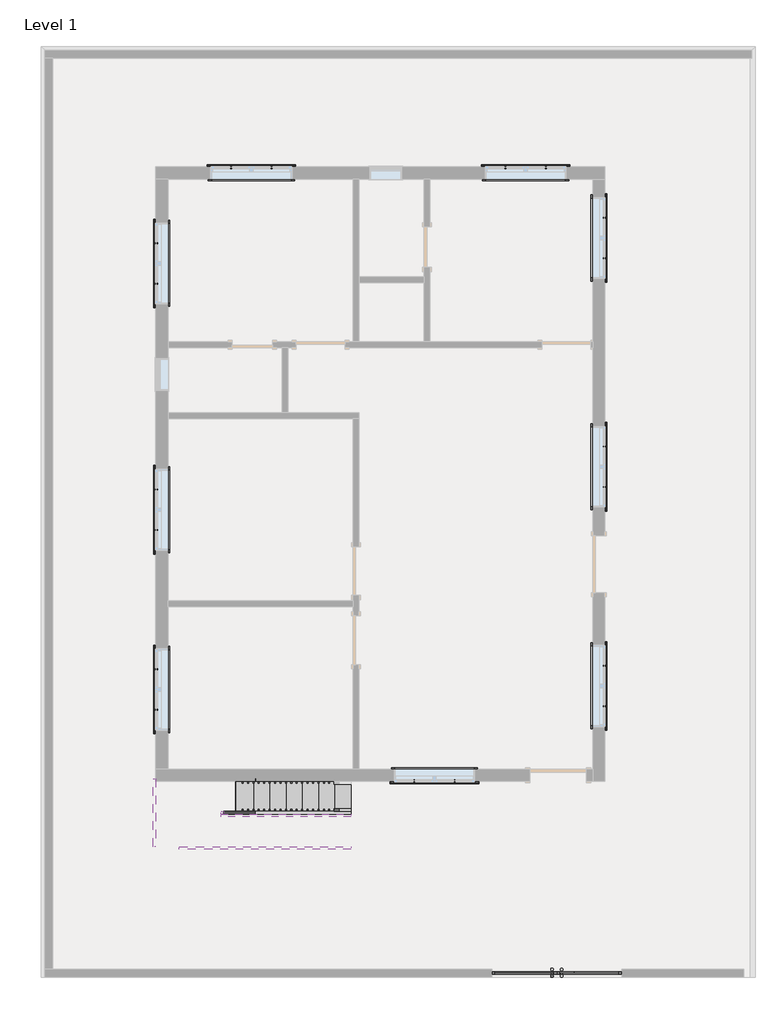
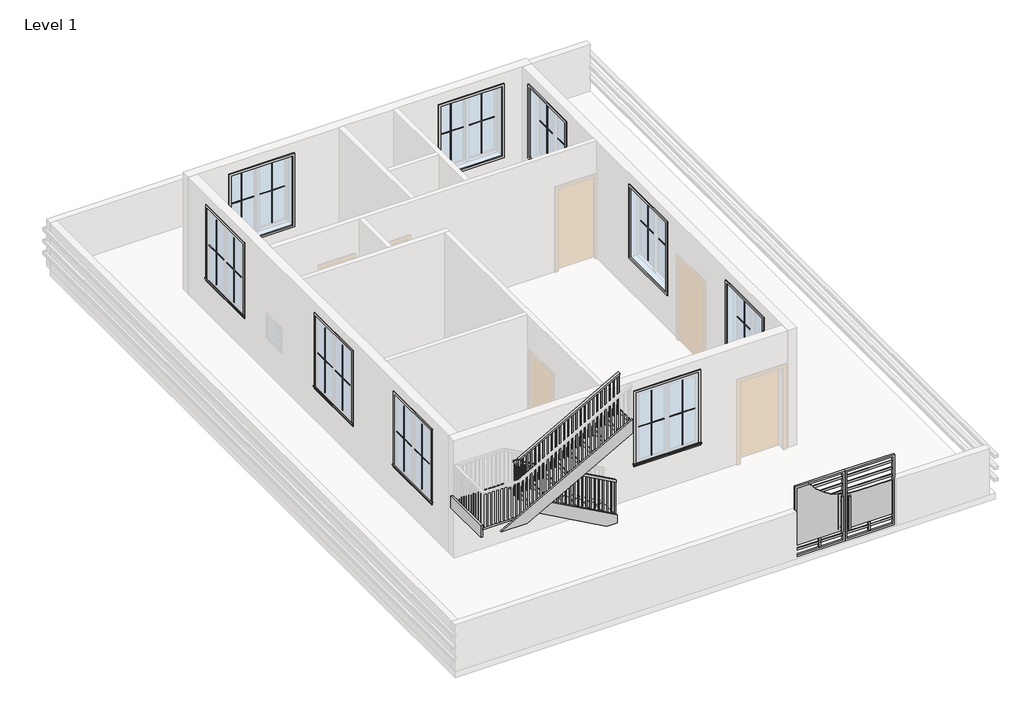
# One storey, part 3 of 3: 37 proxies, 6 members, 1 railing, 1 stair flight.
"""IFC4 building model written with IfcOpenShell, lengths in millimetres."""

from ifc_helpers import new_model, si_unit, frame, origin, place, context, project, spatial, polyline, outline, extrude, faceted_brep, transform, mapped, element, save
from components import generic_models_113f6068, muntin_pattern_2x2_muntin_pattern_2x2_f6a80940, muntin_pattern_2x2_muntin_pattern_2x2_09b00a1c, trim_window_exterior_flat_with_sill_698ed857, trim_window_interior_flat_picture_frame_92551a5e, stair_flight_bb5844b6

model = new_model("IFC4")

# Units and contexts
model_context = context("Model", 3, world=origin())
ifc_project = project(units=[si_unit("LENGTHUNIT", "METRE", prefix="MILLI")], contexts=[model_context])

# Site, building, storey
site = spatial("IfcSite", under=ifc_project)
building = spatial("IfcBuilding", under=site)
storey = spatial("IfcBuildingStorey", under=building, Name="Level 1", Elevation=0.0)

# Proxies
placement = place(None, origin())
generic_models_shape = generic_models_113f6068(model_context)
element("IfcBuildingElementProxy", 1, Name="Generic Models", at=placement, inside=storey, context=model_context, shape_type="MappedRepresentation", body=[
    mapped(generic_models_shape, transform((2054.9561924, -8871.4750537, 0.0), x_axis=(1.0, 0.0, 0.0), y_axis=(0.0, 1.0, 0.0), z_axis=(0.0, 0.0, 1.0))),
])
muntin_pattern_2x2_muntin_pattern_2x2_shape = muntin_pattern_2x2_muntin_pattern_2x2_f6a80940(model_context)
element("IfcBuildingElementProxy", 2, Name="Muntin Pattern_2x2 : Muntin Pattern_2x2", ObjectType="Muntin Pattern_2x2 : Muntin Pattern_2x2", at=placement, inside=storey, context=model_context, shape_type="MappedRepresentation", body=[
    mapped(muntin_pattern_2x2_muntin_pattern_2x2_shape, transform((-5453.9948569, -3961.7808037, 984.25), x_axis=(0.0, 1.0, 0.0), y_axis=(-1.0, 0.0, 0.0), z_axis=(0.0, 0.0, 1.0))),
])
element("IfcBuildingElementProxy", 3, Name="Muntin Pattern_2x2 : Muntin Pattern_2x2", ObjectType="Muntin Pattern_2x2 : Muntin Pattern_2x2", at=placement, inside=storey, context=model_context, shape_type="MappedRepresentation", body=[
    mapped(muntin_pattern_2x2_muntin_pattern_2x2_shape, transform((-5453.9948569, -593.1058037, 984.25), x_axis=(0.0, 1.0, 0.0), y_axis=(-1.0, 0.0, 0.0), z_axis=(0.0, 0.0, 1.0))),
])
element("IfcBuildingElementProxy", 4, Name="Muntin Pattern_2x2 : Muntin Pattern_2x2", ObjectType="Muntin Pattern_2x2 : Muntin Pattern_2x2", at=placement, inside=storey, context=model_context, shape_type="MappedRepresentation", body=[
    mapped(muntin_pattern_2x2_muntin_pattern_2x2_shape, transform((-5453.9948569, 4023.3441963, 984.25), x_axis=(0.0, 1.0, 0.0), y_axis=(-1.0, 0.0, 0.0), z_axis=(0.0, 0.0, 1.0))),
])
element("IfcBuildingElementProxy", 5, Name="Muntin Pattern_2x2 : Muntin Pattern_2x2", ObjectType="Muntin Pattern_2x2 : Muntin Pattern_2x2", at=placement, inside=storey, context=model_context, shape_type="MappedRepresentation", body=[
    mapped(muntin_pattern_2x2_muntin_pattern_2x2_shape, transform((2947.0551431, 5258.4191963, 984.25), x_axis=(0.0, -1.0, 0.0), y_axis=(1.0, 0.0, 0.0), z_axis=(0.0, 0.0, 1.0))),
])
element("IfcBuildingElementProxy", 6, Name="Muntin Pattern_2x2 : Muntin Pattern_2x2", ObjectType="Muntin Pattern_2x2 : Muntin Pattern_2x2", at=placement, inside=storey, context=model_context, shape_type="MappedRepresentation", body=[
    mapped(muntin_pattern_2x2_muntin_pattern_2x2_shape, transform((2947.0551431, 972.1691963, 984.25), x_axis=(0.0, -1.0, 0.0), y_axis=(1.0, 0.0, 0.0), z_axis=(0.0, 0.0, 1.0))),
])
element("IfcBuildingElementProxy", 7, Name="Muntin Pattern_2x2 : Muntin Pattern_2x2", ObjectType="Muntin Pattern_2x2 : Muntin Pattern_2x2", at=placement, inside=storey, context=model_context, shape_type="MappedRepresentation", body=[
    mapped(muntin_pattern_2x2_muntin_pattern_2x2_shape, transform((2947.0551431, -3136.2808037, 984.25), x_axis=(0.0, -1.0, 0.0), y_axis=(1.0, 0.0, 0.0), z_axis=(0.0, 0.0, 1.0))),
])
element("IfcBuildingElementProxy", 8, Name="Muntin Pattern_2x2 : Muntin Pattern_2x2", ObjectType="Muntin Pattern_2x2 : Muntin Pattern_2x2", at=placement, inside=storey, context=model_context, shape_type="MappedRepresentation", body=[
    mapped(muntin_pattern_2x2_muntin_pattern_2x2_shape, transform((141.9426431, -5296.8683037, 984.25), x_axis=(-1.0, 0.0, 0.0), y_axis=(0.0, -1.0, 0.0), z_axis=(0.0, 0.0, 1.0))),
])
element("IfcBuildingElementProxy", 9, Name="Muntin Pattern_2x2 : Muntin Pattern_2x2", ObjectType="Muntin Pattern_2x2 : Muntin Pattern_2x2", at=placement, inside=storey, context=model_context, shape_type="MappedRepresentation", body=[
    mapped(muntin_pattern_2x2_muntin_pattern_2x2_shape, transform((1091.2676431, 6202.9816963, 984.25), x_axis=(1.0, 0.0, 0.0), y_axis=(0.0, 1.0, 0.0), z_axis=(0.0, 0.0, 1.0))),
])
element("IfcBuildingElementProxy", 10, Name="Muntin Pattern_2x2 : Muntin Pattern_2x2", ObjectType="Muntin Pattern_2x2 : Muntin Pattern_2x2", at=placement, inside=storey, context=model_context, shape_type="MappedRepresentation", body=[
    mapped(muntin_pattern_2x2_muntin_pattern_2x2_shape, transform((-4052.2323569, 6202.9816963, 984.25), x_axis=(1.0, 0.0, 0.0), y_axis=(0.0, 1.0, 0.0), z_axis=(0.0, 0.0, 1.0))),
])
muntin_pattern_2x2_muntin_pattern_2x2_2_shape = muntin_pattern_2x2_muntin_pattern_2x2_09b00a1c(model_context)
element("IfcBuildingElementProxy", 11, Name="Muntin Pattern_2x2 : Muntin Pattern_2x2", ObjectType="Muntin Pattern_2x2 : Muntin Pattern_2x2", at=placement, inside=storey, context=model_context, shape_type="MappedRepresentation", body=[
    mapped(muntin_pattern_2x2_muntin_pattern_2x2_2_shape, transform((-5453.9948569, -3202.9558037, 984.25), x_axis=(0.0, -1.0, 0.0), y_axis=(1.0, 0.0, 0.0), z_axis=(0.0, 0.0, 1.0))),
])
element("IfcBuildingElementProxy", 12, Name="Muntin Pattern_2x2 : Muntin Pattern_2x2", ObjectType="Muntin Pattern_2x2 : Muntin Pattern_2x2", at=placement, inside=storey, context=model_context, shape_type="MappedRepresentation", body=[
    mapped(muntin_pattern_2x2_muntin_pattern_2x2_2_shape, transform((-5453.9948569, 165.7191963, 984.25), x_axis=(0.0, -1.0, 0.0), y_axis=(1.0, 0.0, 0.0), z_axis=(0.0, 0.0, 1.0))),
])
element("IfcBuildingElementProxy", 13, Name="Muntin Pattern_2x2 : Muntin Pattern_2x2", ObjectType="Muntin Pattern_2x2 : Muntin Pattern_2x2", at=placement, inside=storey, context=model_context, shape_type="MappedRepresentation", body=[
    mapped(muntin_pattern_2x2_muntin_pattern_2x2_2_shape, transform((-5453.9948569, 4782.1691963, 984.25), x_axis=(0.0, -1.0, 0.0), y_axis=(1.0, 0.0, 0.0), z_axis=(0.0, 0.0, 1.0))),
])
element("IfcBuildingElementProxy", 14, Name="Muntin Pattern_2x2 : Muntin Pattern_2x2", ObjectType="Muntin Pattern_2x2 : Muntin Pattern_2x2", at=placement, inside=storey, context=model_context, shape_type="MappedRepresentation", body=[
    mapped(muntin_pattern_2x2_muntin_pattern_2x2_2_shape, transform((2947.0551431, 4499.5941963, 984.25), x_axis=(0.0, 1.0, 0.0), y_axis=(-1.0, 0.0, 0.0), z_axis=(0.0, 0.0, 1.0))),
])
element("IfcBuildingElementProxy", 15, Name="Muntin Pattern_2x2 : Muntin Pattern_2x2", ObjectType="Muntin Pattern_2x2 : Muntin Pattern_2x2", at=placement, inside=storey, context=model_context, shape_type="MappedRepresentation", body=[
    mapped(muntin_pattern_2x2_muntin_pattern_2x2_2_shape, transform((2947.0551431, 213.3441963, 984.25), x_axis=(0.0, 1.0, 0.0), y_axis=(-1.0, 0.0, 0.0), z_axis=(0.0, 0.0, 1.0))),
])
element("IfcBuildingElementProxy", 16, Name="Muntin Pattern_2x2 : Muntin Pattern_2x2", ObjectType="Muntin Pattern_2x2 : Muntin Pattern_2x2", at=placement, inside=storey, context=model_context, shape_type="MappedRepresentation", body=[
    mapped(muntin_pattern_2x2_muntin_pattern_2x2_2_shape, transform((2947.0551431, -3895.1058037, 984.25), x_axis=(0.0, 1.0, 0.0), y_axis=(-1.0, 0.0, 0.0), z_axis=(0.0, 0.0, 1.0))),
])
element("IfcBuildingElementProxy", 17, Name="Muntin Pattern_2x2 : Muntin Pattern_2x2", ObjectType="Muntin Pattern_2x2 : Muntin Pattern_2x2", at=placement, inside=storey, context=model_context, shape_type="MappedRepresentation", body=[
    mapped(muntin_pattern_2x2_muntin_pattern_2x2_2_shape, transform((-616.8823569, -5296.8683037, 984.25), x_axis=(1.0, 0.0, 0.0), y_axis=(0.0, 1.0, 0.0), z_axis=(0.0, 0.0, 1.0))),
])
element("IfcBuildingElementProxy", 18, Name="Muntin Pattern_2x2 : Muntin Pattern_2x2", ObjectType="Muntin Pattern_2x2 : Muntin Pattern_2x2", at=placement, inside=storey, context=model_context, shape_type="MappedRepresentation", body=[
    mapped(muntin_pattern_2x2_muntin_pattern_2x2_2_shape, transform((1850.0926431, 6202.9816963, 984.25), x_axis=(-1.0, 0.0, 0.0), y_axis=(0.0, -1.0, 0.0), z_axis=(0.0, 0.0, 1.0))),
])
element("IfcBuildingElementProxy", 19, Name="Muntin Pattern_2x2 : Muntin Pattern_2x2", ObjectType="Muntin Pattern_2x2 : Muntin Pattern_2x2", at=placement, inside=storey, context=model_context, shape_type="MappedRepresentation", body=[
    mapped(muntin_pattern_2x2_muntin_pattern_2x2_2_shape, transform((-3293.4073569, 6202.9816963, 984.25), x_axis=(-1.0, 0.0, 0.0), y_axis=(0.0, -1.0, 0.0), z_axis=(0.0, 0.0, 1.0))),
])
trim_window_exterior_flat_with_sill_shape = trim_window_exterior_flat_with_sill_698ed857(model_context)
element("IfcBuildingElementProxy", 20, Name="Trim-Window-Exterior-Flat : with Sill", ObjectType="Trim-Window-Exterior-Flat : with Sill", at=placement, inside=storey, context=model_context, shape_type="MappedRepresentation", body=[
    mapped(trim_window_exterior_flat_with_sill_shape, transform((-5463.5198569, -3582.3683037, 2743.2), x_axis=(0.0, -1.0, 0.0), y_axis=(0.0, 0.0, 1.0), z_axis=(-1.0, 0.0, 0.0))),
])
element("IfcBuildingElementProxy", 21, Name="Trim-Window-Exterior-Flat : with Sill", ObjectType="Trim-Window-Exterior-Flat : with Sill", at=placement, inside=storey, context=model_context, shape_type="MappedRepresentation", body=[
    mapped(trim_window_exterior_flat_with_sill_shape, transform((-5463.5198569, -213.6933037, 2743.2), x_axis=(0.0, -1.0, 0.0), y_axis=(0.0, 0.0, 1.0), z_axis=(-1.0, 0.0, 0.0))),
])
element("IfcBuildingElementProxy", 22, Name="Trim-Window-Exterior-Flat : with Sill", ObjectType="Trim-Window-Exterior-Flat : with Sill", at=placement, inside=storey, context=model_context, shape_type="MappedRepresentation", body=[
    mapped(trim_window_exterior_flat_with_sill_shape, transform((-5463.5198569, 4402.7566963, 2743.2), x_axis=(0.0, -1.0, 0.0), y_axis=(0.0, 0.0, 1.0), z_axis=(-1.0, 0.0, 0.0))),
])
element("IfcBuildingElementProxy", 23, Name="Trim-Window-Exterior-Flat : with Sill", ObjectType="Trim-Window-Exterior-Flat : with Sill", at=placement, inside=storey, context=model_context, shape_type="MappedRepresentation", body=[
    mapped(trim_window_exterior_flat_with_sill_shape, transform((2956.5801431, 4879.0066963, 2743.2), x_axis=(0.0, 1.0, 0.0), y_axis=(0.0, 0.0, 1.0), z_axis=(1.0, 0.0, 0.0))),
])
element("IfcBuildingElementProxy", 24, Name="Trim-Window-Exterior-Flat : with Sill", ObjectType="Trim-Window-Exterior-Flat : with Sill", at=placement, inside=storey, context=model_context, shape_type="MappedRepresentation", body=[
    mapped(trim_window_exterior_flat_with_sill_shape, transform((2956.5801431, 592.7566963, 2743.2), x_axis=(0.0, 1.0, 0.0), y_axis=(0.0, 0.0, 1.0), z_axis=(1.0, 0.0, 0.0))),
])
element("IfcBuildingElementProxy", 25, Name="Trim-Window-Exterior-Flat : with Sill", ObjectType="Trim-Window-Exterior-Flat : with Sill", at=placement, inside=storey, context=model_context, shape_type="MappedRepresentation", body=[
    mapped(trim_window_exterior_flat_with_sill_shape, transform((2956.5801431, -3515.6933037, 2743.2), x_axis=(0.0, 1.0, 0.0), y_axis=(0.0, 0.0, 1.0), z_axis=(1.0, 0.0, 0.0))),
])
element("IfcBuildingElementProxy", 26, Name="Trim-Window-Exterior-Flat : with Sill", ObjectType="Trim-Window-Exterior-Flat : with Sill", at=placement, inside=storey, context=model_context, shape_type="MappedRepresentation", body=[
    mapped(trim_window_exterior_flat_with_sill_shape, transform((-237.4698569, -5306.3933037, 2743.2), x_axis=(1.0, 0.0, 0.0), y_axis=(0.0, 0.0, 1.0), z_axis=(0.0, -1.0, 0.0))),
])
element("IfcBuildingElementProxy", 27, Name="Trim-Window-Exterior-Flat : with Sill", ObjectType="Trim-Window-Exterior-Flat : with Sill", at=placement, inside=storey, context=model_context, shape_type="MappedRepresentation", body=[
    mapped(trim_window_exterior_flat_with_sill_shape, transform((1470.6801431, 6212.5066963, 2743.2), x_axis=(-1.0, 0.0, 0.0), y_axis=(0.0, 0.0, 1.0), z_axis=(0.0, 1.0, 0.0))),
])
element("IfcBuildingElementProxy", 28, Name="Trim-Window-Exterior-Flat : with Sill", ObjectType="Trim-Window-Exterior-Flat : with Sill", at=placement, inside=storey, context=model_context, shape_type="MappedRepresentation", body=[
    mapped(trim_window_exterior_flat_with_sill_shape, transform((-3672.8198569, 6212.5066963, 2743.2), x_axis=(-1.0, 0.0, 0.0), y_axis=(0.0, 0.0, 1.0), z_axis=(0.0, 1.0, 0.0))),
])
trim_window_interior_flat_picture_frame_shape = trim_window_interior_flat_picture_frame_92551a5e(model_context)
element("IfcBuildingElementProxy", 29, Name="Trim-Window-Interior-Flat : Picture Frame", ObjectType="Trim-Window-Interior-Flat : Picture Frame", at=placement, inside=storey, context=model_context, shape_type="MappedRepresentation", body=[
    mapped(trim_window_interior_flat_picture_frame_shape, transform((-5234.9198569, -3582.3683037, 2743.2), x_axis=(0.0, 1.0, 0.0), y_axis=(0.0, 0.0, 1.0), z_axis=(1.0, 0.0, 0.0))),
])
element("IfcBuildingElementProxy", 30, Name="Trim-Window-Interior-Flat : Picture Frame", ObjectType="Trim-Window-Interior-Flat : Picture Frame", at=placement, inside=storey, context=model_context, shape_type="MappedRepresentation", body=[
    mapped(trim_window_interior_flat_picture_frame_shape, transform((-5234.9198569, -213.6933037, 2743.2), x_axis=(0.0, 1.0, 0.0), y_axis=(0.0, 0.0, 1.0), z_axis=(1.0, 0.0, 0.0))),
])
element("IfcBuildingElementProxy", 31, Name="Trim-Window-Interior-Flat : Picture Frame", ObjectType="Trim-Window-Interior-Flat : Picture Frame", at=placement, inside=storey, context=model_context, shape_type="MappedRepresentation", body=[
    mapped(trim_window_interior_flat_picture_frame_shape, transform((-5234.9198569, 4402.7566963, 2743.2), x_axis=(0.0, 1.0, 0.0), y_axis=(0.0, 0.0, 1.0), z_axis=(1.0, 0.0, 0.0))),
])
element("IfcBuildingElementProxy", 32, Name="Trim-Window-Interior-Flat : Picture Frame", ObjectType="Trim-Window-Interior-Flat : Picture Frame", at=placement, inside=storey, context=model_context, shape_type="MappedRepresentation", body=[
    mapped(trim_window_interior_flat_picture_frame_shape, transform((2727.9801431, 4879.0066963, 2743.2), x_axis=(0.0, -1.0, 0.0), y_axis=(0.0, 0.0, 1.0), z_axis=(-1.0, 0.0, 0.0))),
])
element("IfcBuildingElementProxy", 33, Name="Trim-Window-Interior-Flat : Picture Frame", ObjectType="Trim-Window-Interior-Flat : Picture Frame", at=placement, inside=storey, context=model_context, shape_type="MappedRepresentation", body=[
    mapped(trim_window_interior_flat_picture_frame_shape, transform((2727.9801431, 592.7566963, 2743.2), x_axis=(0.0, -1.0, 0.0), y_axis=(0.0, 0.0, 1.0), z_axis=(-1.0, 0.0, 0.0))),
])
element("IfcBuildingElementProxy", 34, Name="Trim-Window-Interior-Flat : Picture Frame", ObjectType="Trim-Window-Interior-Flat : Picture Frame", at=placement, inside=storey, context=model_context, shape_type="MappedRepresentation", body=[
    mapped(trim_window_interior_flat_picture_frame_shape, transform((2727.9801431, -3515.6933037, 2743.2), x_axis=(0.0, -1.0, 0.0), y_axis=(0.0, 0.0, 1.0), z_axis=(-1.0, 0.0, 0.0))),
])
element("IfcBuildingElementProxy", 35, Name="Trim-Window-Interior-Flat : Picture Frame", ObjectType="Trim-Window-Interior-Flat : Picture Frame", at=placement, inside=storey, context=model_context, shape_type="MappedRepresentation", body=[
    mapped(trim_window_interior_flat_picture_frame_shape, transform((-237.4698569, -5077.7933037, 2743.2), x_axis=(-1.0, 0.0, 0.0), y_axis=(0.0, 0.0, 1.0), z_axis=(0.0, 1.0, 0.0))),
])
element("IfcBuildingElementProxy", 36, Name="Trim-Window-Interior-Flat : Picture Frame", ObjectType="Trim-Window-Interior-Flat : Picture Frame", at=placement, inside=storey, context=model_context, shape_type="MappedRepresentation", body=[
    mapped(trim_window_interior_flat_picture_frame_shape, transform((1470.6801431, 5983.9066963, 2743.2), x_axis=(1.0, 0.0, 0.0), y_axis=(0.0, 0.0, 1.0), z_axis=(0.0, -1.0, 0.0))),
])
element("IfcBuildingElementProxy", 37, Name="Trim-Window-Interior-Flat : Picture Frame", ObjectType="Trim-Window-Interior-Flat : Picture Frame", at=placement, inside=storey, context=model_context, shape_type="MappedRepresentation", body=[
    mapped(trim_window_interior_flat_picture_frame_shape, transform((-3672.8198569, 5983.9066963, 2743.2), x_axis=(1.0, 0.0, 0.0), y_axis=(0.0, 0.0, 1.0), z_axis=(0.0, -1.0, 0.0))),
])

# Members
element("IfcMember", 38, ObjectType="Stringer - 2\" Width", at=placement, inside=storey, context=model_context, shape_type="SweptSolid", body=[
    extrude(outline(polyline([(0.0, -1805.9198569), (207.5983948, -1805.9198569), (1534.0428392, -4193.5198569), (1185.3641651, -4193.5198569), (0.0, -2059.8643597), (0.0, -1805.9198569)])), frame((0.0, -5915.9933037, 0.0), z_axis=(0.0, 1.0, 0.0), x_axis=(0.0, 0.0, 1.0)), (0.0, 0.0, 1.0), 50.8),
])
element("IfcMember", 39, ObjectType="Stringer - 2\" Width", at=placement, inside=storey, context=model_context, shape_type="SweptSolid", body=[
    extrude(outline(polyline([(-4244.3198569, -5865.1933037), (-4193.5198569, -5865.1933037), (-4193.5198569, -5915.9933037), (-4244.3198569, -5915.9933037), (-4244.3198569, -5865.1933037)])), frame((0.0, 0.0, 1295.4), z_axis=(0.0, 0.0, 1.0), x_axis=(1.0, 0.0, 0.0)), (0.0, 0.0, 1.0), 304.8),
])
element("IfcMember", 40, ObjectType="Stringer - 2\" Width", at=placement, inside=storey, context=model_context, shape_type="SweptSolid", body=[
    extrude(outline(polyline([(1731.5983948, -4244.3198569), (1382.9197207, -4244.3198569), (2737.5863873, -1805.9198569), (3086.2650614, -1805.9198569), (1731.5983948, -4244.3198569)])), frame((0.0, -5966.7933037, 0.0), z_axis=(0.0, 1.0, 0.0), x_axis=(0.0, 0.0, 1.0)), (0.0, 0.0, 1.0), 50.8),
])
element("IfcMember", 41, ObjectType="Stringer - 2\" Width", at=placement, inside=storey, context=model_context, shape_type="SweptSolid", body=[
    extrude(outline(polyline([(0.0, -1805.9198569), (207.5983948, -1805.9198569), (1600.2, -4312.6027463), (1600.2, -4940.2243597), (0.0, -2059.8643597), (0.0, -1805.9198569)])), frame((0.0, -5306.3933037, 0.0), z_axis=(0.0, 1.0, 0.0), x_axis=(0.0, 0.0, 1.0)), (0.0, 0.0, 1.0), 50.8),
])
element("IfcMember", 42, ObjectType="Stringer - 2\" Width", at=placement, inside=storey, context=model_context, shape_type="SweptSolid", body=[
    extrude(outline(polyline([(-5514.3198569, -5255.5933037), (-5463.5198569, -5255.5933037), (-5463.5198569, -6525.5933037), (-5514.3198569, -6525.5933037), (-5514.3198569, -5255.5933037)])), frame((0.0, 0.0, 1295.4), z_axis=(0.0, 0.0, 1.0), x_axis=(1.0, 0.0, 0.0)), (0.0, 0.0, 1.0), 304.8),
])
element("IfcMember", 43, ObjectType="Stringer - 2\" Width", at=placement, inside=storey, context=model_context, shape_type="SweptSolid", body=[
    extrude(outline(polyline([(1295.4, -4401.8553541), (2737.5863873, -1805.9198569), (3086.2650614, -1805.9198569), (1295.4, -5029.4769675), (1295.4, -4401.8553541)])), frame((0.0, -6576.3933037, 0.0), z_axis=(0.0, 1.0, 0.0), x_axis=(0.0, 0.0, 1.0)), (0.0, 0.0, 1.0), 50.8),
])

# Railing
element("IfcRailing", 44, ObjectType="Handrail - Rectangular", at=placement, inside=storey, context=model_context, shape_type="SolidModel", body=[
    faceted_brep([(-1805.9198569, -5865.1933037, 1083.7333333), (-1805.9198569, -5865.1933037, 1025.620221), (-1805.9198569, -5814.3933037, 1025.620221), (-1805.9198569, -5814.3933037, 1083.7333333), (-4168.1198569, -5865.1933037, 2396.0666667), (-4218.9198569, -5865.1933037, 2366.1757765), (-4218.9198569, -5814.3933037, 2366.1757765), (-4168.1198569, -5814.3933037, 2396.0666667), (-4168.1198569, -5865.1933037, 2438.4), (-4218.9198569, -5865.1933037, 2387.6), (-4218.9198569, -5814.3933037, 2387.6), (-4168.1198569, -5814.3933037, 2438.4), (-4244.3198569, -5865.1933037, 2438.4), (-4244.3198569, -5865.1933037, 2387.6), (-4295.1198569, -5814.3933037, 2387.6), (-4295.1198569, -5814.3933037, 2438.4), (-4244.3198569, -5941.3933037, 2438.4), (-4244.3198569, -5941.3933037, 2387.6), (-4295.1198569, -5941.3933037, 2387.6), (-4295.1198569, -5941.3933037, 2438.4), (-4244.3198569, -5966.7933037, 2438.4), (-4295.1198569, -5966.7933037, 2438.4), (-4295.1198569, -6017.5933037, 2387.6), (-4244.3198569, -6017.5933037, 2387.6)], [[[0, 1, 2, 3]], [[1, 0, 4, 5]], [[2, 1, 5, 6]], [[3, 2, 6, 7]], [[0, 3, 7, 4]], [[5, 4, 8, 9]], [[6, 5, 9, 10]], [[7, 6, 10, 11]], [[4, 7, 11, 8]], [[9, 8, 12, 13]], [[10, 9, 13, 14]], [[11, 10, 14, 15]], [[8, 11, 15, 12]], [[13, 12, 16, 17]], [[14, 13, 17, 18]], [[15, 14, 18, 19]], [[12, 15, 19, 16]], [[20, 21, 22, 23]], [[17, 16, 20, 23]], [[18, 17, 23, 22]], [[19, 18, 22, 21]], [[16, 19, 21, 20]]]),
    faceted_brep([(-4244.3198569, -5966.7933037, 2438.4), (-4244.3198569, -6017.5933037, 2387.6), (-4295.1198569, -6017.5933037, 2387.6), (-4295.1198569, -5966.7933037, 2438.4), (-4244.3198569, -5966.7933037, 2549.620221), (-4295.1198569, -5966.7933037, 2579.5111111), (-4295.1198569, -6017.5933037, 2579.5111111), (-4244.3198569, -6017.5933037, 2549.620221)], [[[0, 1, 2, 3]], [[4, 5, 6, 7]], [[1, 0, 4, 7]], [[2, 1, 7, 6]], [[3, 2, 6, 5]], [[0, 3, 5, 4]]]),
    faceted_brep([(-4295.1198569, -5966.7933037, 2579.5111111), (-4244.3198569, -5966.7933037, 2549.620221), (-4244.3198569, -6017.5933037, 2549.620221), (-4295.1198569, -6017.5933037, 2579.5111111), (-1805.9198569, -5966.7933037, 3962.4), (-1805.9198569, -6017.5933037, 3962.4), (-1805.9198569, -6017.5933037, 3904.2868876), (-1805.9198569, -5966.7933037, 3904.2868876)], [[[0, 1, 2, 3]], [[4, 5, 6, 7]], [[1, 0, 4, 7]], [[2, 1, 7, 6]], [[3, 2, 6, 5]], [[0, 3, 5, 4]]]),
    extrude(outline(polyline([(3884.8841099, -1840.8448569), (2878.6666667, -1840.8448569), (2878.6666667, -1821.7948569), (3895.4674432, -1821.7948569), (3884.8841099, -1840.8448569)])), frame((0.0, -6001.7183037, 0.0), z_axis=(0.0, 1.0, 0.0), x_axis=(0.0, 0.0, 1.0)), (0.0, 0.0, 1.0), 19.05),
    extrude(outline(polyline([(3828.4396654, -1942.4448569), (2878.6666667, -1942.4448569), (2878.6666667, -1923.3948569), (3839.0229988, -1923.3948569), (3828.4396654, -1942.4448569)])), frame((0.0, -6001.7183037, 0.0), z_axis=(0.0, 1.0, 0.0), x_axis=(0.0, 0.0, 1.0)), (0.0, 0.0, 1.0), 19.05),
    extrude(outline(polyline([(3771.995221, -2044.0448569), (2878.6666667, -2044.0448569), (2878.6666667, -2024.9948569), (3782.5785543, -2024.9948569), (3771.995221, -2044.0448569)])), frame((0.0, -6001.7183037, 0.0), z_axis=(0.0, 1.0, 0.0), x_axis=(0.0, 0.0, 1.0)), (0.0, 0.0, 1.0), 19.05),
    extrude(outline(polyline([(3715.5507765, -2145.6448569), (2709.3333333, -2145.6448569), (2709.3333333, -2126.5948569), (3726.1341099, -2126.5948569), (3715.5507765, -2145.6448569)])), frame((0.0, -6001.7183037, 0.0), z_axis=(0.0, 1.0, 0.0), x_axis=(0.0, 0.0, 1.0)), (0.0, 0.0, 1.0), 19.05),
    extrude(outline(polyline([(3659.1063321, -2247.2448569), (2709.3333333, -2247.2448569), (2709.3333333, -2228.1948569), (3669.6896654, -2228.1948569), (3659.1063321, -2247.2448569)])), frame((0.0, -6001.7183037, 0.0), z_axis=(0.0, 1.0, 0.0), x_axis=(0.0, 0.0, 1.0)), (0.0, 0.0, 1.0), 19.05),
    extrude(outline(polyline([(3602.6618876, -2348.8448569), (2709.3333333, -2348.8448569), (2709.3333333, -2329.7948569), (3613.245221, -2329.7948569), (3602.6618876, -2348.8448569)])), frame((0.0, -6001.7183037, 0.0), z_axis=(0.0, 1.0, 0.0), x_axis=(0.0, 0.0, 1.0)), (0.0, 0.0, 1.0), 19.05),
    extrude(outline(polyline([(3546.2174432, -2450.4448569), (2540.0, -2450.4448569), (2540.0, -2431.3948569), (3556.8007765, -2431.3948569), (3546.2174432, -2450.4448569)])), frame((0.0, -6001.7183037, 0.0), z_axis=(0.0, 1.0, 0.0), x_axis=(0.0, 0.0, 1.0)), (0.0, 0.0, 1.0), 19.05),
    extrude(outline(polyline([(3489.7729988, -2552.0448569), (2540.0, -2552.0448569), (2540.0, -2532.9948569), (3500.3563321, -2532.9948569), (3489.7729988, -2552.0448569)])), frame((0.0, -6001.7183037, 0.0), z_axis=(0.0, 1.0, 0.0), x_axis=(0.0, 0.0, 1.0)), (0.0, 0.0, 1.0), 19.05),
    extrude(outline(polyline([(3433.3285543, -2653.6448569), (2540.0, -2653.6448569), (2540.0, -2634.5948569), (3443.9118876, -2634.5948569), (3433.3285543, -2653.6448569)])), frame((0.0, -6001.7183037, 0.0), z_axis=(0.0, 1.0, 0.0), x_axis=(0.0, 0.0, 1.0)), (0.0, 0.0, 1.0), 19.05),
    extrude(outline(polyline([(3376.8841099, -2755.2448569), (2370.6666667, -2755.2448569), (2370.6666667, -2736.1948569), (3387.4674432, -2736.1948569), (3376.8841099, -2755.2448569)])), frame((0.0, -6001.7183037, 0.0), z_axis=(0.0, 1.0, 0.0), x_axis=(0.0, 0.0, 1.0)), (0.0, 0.0, 1.0), 19.05),
    extrude(outline(polyline([(3320.4396654, -2856.8448569), (2370.6666667, -2856.8448569), (2370.6666667, -2837.7948569), (3331.0229988, -2837.7948569), (3320.4396654, -2856.8448569)])), frame((0.0, -6001.7183037, 0.0), z_axis=(0.0, 1.0, 0.0), x_axis=(0.0, 0.0, 1.0)), (0.0, 0.0, 1.0), 19.05),
    extrude(outline(polyline([(3263.995221, -2958.4448569), (2370.6666667, -2958.4448569), (2370.6666667, -2939.3948569), (3274.5785543, -2939.3948569), (3263.995221, -2958.4448569)])), frame((0.0, -6001.7183037, 0.0), z_axis=(0.0, 1.0, 0.0), x_axis=(0.0, 0.0, 1.0)), (0.0, 0.0, 1.0), 19.05),
    extrude(outline(polyline([(3207.5507765, -3060.0448569), (2201.3333333, -3060.0448569), (2201.3333333, -3040.9948569), (3218.1341099, -3040.9948569), (3207.5507765, -3060.0448569)])), frame((0.0, -6001.7183037, 0.0), z_axis=(0.0, 1.0, 0.0), x_axis=(0.0, 0.0, 1.0)), (0.0, 0.0, 1.0), 19.05),
    extrude(outline(polyline([(3151.1063321, -3161.6448569), (2201.3333333, -3161.6448569), (2201.3333333, -3142.5948569), (3161.6896654, -3142.5948569), (3151.1063321, -3161.6448569)])), frame((0.0, -6001.7183037, 0.0), z_axis=(0.0, 1.0, 0.0), x_axis=(0.0, 0.0, 1.0)), (0.0, 0.0, 1.0), 19.05),
    extrude(outline(polyline([(3094.6618876, -3263.2448569), (2201.3333333, -3263.2448569), (2201.3333333, -3244.1948569), (3105.245221, -3244.1948569), (3094.6618876, -3263.2448569)])), frame((0.0, -6001.7183037, 0.0), z_axis=(0.0, 1.0, 0.0), x_axis=(0.0, 0.0, 1.0)), (0.0, 0.0, 1.0), 19.05),
    extrude(outline(polyline([(3038.2174432, -3364.8448569), (2032.0, -3364.8448569), (2032.0, -3345.7948569), (3048.8007765, -3345.7948569), (3038.2174432, -3364.8448569)])), frame((0.0, -6001.7183037, 0.0), z_axis=(0.0, 1.0, 0.0), x_axis=(0.0, 0.0, 1.0)), (0.0, 0.0, 1.0), 19.05),
    extrude(outline(polyline([(2981.7729988, -3466.4448569), (2032.0, -3466.4448569), (2032.0, -3447.3948569), (2992.3563321, -3447.3948569), (2981.7729988, -3466.4448569)])), frame((0.0, -6001.7183037, 0.0), z_axis=(0.0, 1.0, 0.0), x_axis=(0.0, 0.0, 1.0)), (0.0, 0.0, 1.0), 19.05),
    extrude(outline(polyline([(2925.3285543, -3568.0448569), (2032.0, -3568.0448569), (2032.0, -3548.9948569), (2935.9118876, -3548.9948569), (2925.3285543, -3568.0448569)])), frame((0.0, -6001.7183037, 0.0), z_axis=(0.0, 1.0, 0.0), x_axis=(0.0, 0.0, 1.0)), (0.0, 0.0, 1.0), 19.05),
    extrude(outline(polyline([(2868.8841099, -3669.6448569), (1862.6666667, -3669.6448569), (1862.6666667, -3650.5948569), (2879.4674432, -3650.5948569), (2868.8841099, -3669.6448569)])), frame((0.0, -6001.7183037, 0.0), z_axis=(0.0, 1.0, 0.0), x_axis=(0.0, 0.0, 1.0)), (0.0, 0.0, 1.0), 19.05),
    extrude(outline(polyline([(2812.4396654, -3771.2448569), (1862.6666667, -3771.2448569), (1862.6666667, -3752.1948569), (2823.0229988, -3752.1948569), (2812.4396654, -3771.2448569)])), frame((0.0, -6001.7183037, 0.0), z_axis=(0.0, 1.0, 0.0), x_axis=(0.0, 0.0, 1.0)), (0.0, 0.0, 1.0), 19.05),
    extrude(outline(polyline([(2755.995221, -3872.8448569), (1862.6666667, -3872.8448569), (1862.6666667, -3853.7948569), (2766.5785543, -3853.7948569), (2755.995221, -3872.8448569)])), frame((0.0, -6001.7183037, 0.0), z_axis=(0.0, 1.0, 0.0), x_axis=(0.0, 0.0, 1.0)), (0.0, 0.0, 1.0), 19.05),
    extrude(outline(polyline([(2699.5507765, -3974.4448569), (1693.3333333, -3974.4448569), (1693.3333333, -3955.3948569), (2710.1341099, -3955.3948569), (2699.5507765, -3974.4448569)])), frame((0.0, -6001.7183037, 0.0), z_axis=(0.0, 1.0, 0.0), x_axis=(0.0, 0.0, 1.0)), (0.0, 0.0, 1.0), 19.05),
    extrude(outline(polyline([(2643.1063321, -4076.0448569), (1693.3333333, -4076.0448569), (1693.3333333, -4056.9948569), (2653.6896654, -4056.9948569), (2643.1063321, -4076.0448569)])), frame((0.0, -6001.7183037, 0.0), z_axis=(0.0, 1.0, 0.0), x_axis=(0.0, 0.0, 1.0)), (0.0, 0.0, 1.0), 19.05),
    extrude(outline(polyline([(2586.6618876, -4177.6448569), (1693.3333333, -4177.6448569), (1693.3333333, -4158.5948569), (2597.245221, -4158.5948569), (2586.6618876, -4177.6448569)])), frame((0.0, -6001.7183037, 0.0), z_axis=(0.0, 1.0, 0.0), x_axis=(0.0, 0.0, 1.0)), (0.0, 0.0, 1.0), 19.05),
    extrude(outline(polyline([(-4260.1948569, -5931.8683037), (-4260.1948569, -5950.9183037), (-4279.2448569, -5950.9183037), (-4279.2448569, -5931.8683037), (-4260.1948569, -5931.8683037)])), frame((0.0, 0.0, 1524.0), z_axis=(0.0, 0.0, 1.0), x_axis=(1.0, 0.0, 0.0)), (0.0, 0.0, 1.0), 863.6),
    extrude(outline(polyline([(-4234.7948569, -5849.3183037), (-4253.8448569, -5849.3183037), (-4253.8448569, -5830.2683037), (-4234.7948569, -5830.2683037), (-4234.7948569, -5849.3183037)])), frame((0.0, 0.0, 1524.0), z_axis=(0.0, 0.0, 1.0), x_axis=(1.0, 0.0, 0.0)), (0.0, 0.0, 1.0), 863.6),
    extrude(outline(polyline([(2329.1341099, -4152.2448569), (1354.6666667, -4152.2448569), (1354.6666667, -4133.1948569), (2318.5507765, -4133.1948569), (2329.1341099, -4152.2448569)])), frame((0.0, -5849.3183037, 0.0), z_axis=(0.0, 1.0, 0.0), x_axis=(0.0, 0.0, 1.0)), (0.0, 0.0, 1.0), 19.05),
    extrude(outline(polyline([(2272.6896654, -4050.6448569), (1354.6666667, -4050.6448569), (1354.6666667, -4031.5948569), (2262.1063321, -4031.5948569), (2272.6896654, -4050.6448569)])), frame((0.0, -5849.3183037, 0.0), z_axis=(0.0, 1.0, 0.0), x_axis=(0.0, 0.0, 1.0)), (0.0, 0.0, 1.0), 19.05),
    extrude(outline(polyline([(2216.245221, -3949.0448569), (1354.6666667, -3949.0448569), (1354.6666667, -3929.9948569), (2205.6618876, -3929.9948569), (2216.245221, -3949.0448569)])), frame((0.0, -5849.3183037, 0.0), z_axis=(0.0, 1.0, 0.0), x_axis=(0.0, 0.0, 1.0)), (0.0, 0.0, 1.0), 19.05),
    extrude(outline(polyline([(2159.8007765, -3847.4448569), (1185.3333333, -3847.4448569), (1185.3333333, -3828.3948569), (2149.2174432, -3828.3948569), (2159.8007765, -3847.4448569)])), frame((0.0, -5849.3183037, 0.0), z_axis=(0.0, 1.0, 0.0), x_axis=(0.0, 0.0, 1.0)), (0.0, 0.0, 1.0), 19.05),
    extrude(outline(polyline([(2103.3563321, -3745.8448569), (1185.3333333, -3745.8448569), (1185.3333333, -3726.7948569), (2092.7729988, -3726.7948569), (2103.3563321, -3745.8448569)])), frame((0.0, -5849.3183037, 0.0), z_axis=(0.0, 1.0, 0.0), x_axis=(0.0, 0.0, 1.0)), (0.0, 0.0, 1.0), 19.05),
    extrude(outline(polyline([(2046.9118876, -3644.2448569), (1185.3333333, -3644.2448569), (1185.3333333, -3625.1948569), (2036.3285543, -3625.1948569), (2046.9118876, -3644.2448569)])), frame((0.0, -5849.3183037, 0.0), z_axis=(0.0, 1.0, 0.0), x_axis=(0.0, 0.0, 1.0)), (0.0, 0.0, 1.0), 19.05),
    extrude(outline(polyline([(1990.4674432, -3542.6448569), (1016.0, -3542.6448569), (1016.0, -3523.5948569), (1979.8841099, -3523.5948569), (1990.4674432, -3542.6448569)])), frame((0.0, -5849.3183037, 0.0), z_axis=(0.0, 1.0, 0.0), x_axis=(0.0, 0.0, 1.0)), (0.0, 0.0, 1.0), 19.05),
    extrude(outline(polyline([(1934.0229988, -3441.0448569), (1016.0, -3441.0448569), (1016.0, -3421.9948569), (1923.4396654, -3421.9948569), (1934.0229988, -3441.0448569)])), frame((0.0, -5849.3183037, 0.0), z_axis=(0.0, 1.0, 0.0), x_axis=(0.0, 0.0, 1.0)), (0.0, 0.0, 1.0), 19.05),
    extrude(outline(polyline([(1877.5785543, -3339.4448569), (1016.0, -3339.4448569), (1016.0, -3320.3948569), (1866.995221, -3320.3948569), (1877.5785543, -3339.4448569)])), frame((0.0, -5849.3183037, 0.0), z_axis=(0.0, 1.0, 0.0), x_axis=(0.0, 0.0, 1.0)), (0.0, 0.0, 1.0), 19.05),
    extrude(outline(polyline([(1821.1341099, -3237.8448569), (846.6666667, -3237.8448569), (846.6666667, -3218.7948569), (1810.5507765, -3218.7948569), (1821.1341099, -3237.8448569)])), frame((0.0, -5849.3183037, 0.0), z_axis=(0.0, 1.0, 0.0), x_axis=(0.0, 0.0, 1.0)), (0.0, 0.0, 1.0), 19.05),
    extrude(outline(polyline([(1764.6896654, -3136.2448569), (846.6666667, -3136.2448569), (846.6666667, -3117.1948569), (1754.1063321, -3117.1948569), (1764.6896654, -3136.2448569)])), frame((0.0, -5849.3183037, 0.0), z_axis=(0.0, 1.0, 0.0), x_axis=(0.0, 0.0, 1.0)), (0.0, 0.0, 1.0), 19.05),
    extrude(outline(polyline([(1708.245221, -3034.6448569), (846.6666667, -3034.6448569), (846.6666667, -3015.5948569), (1697.6618876, -3015.5948569), (1708.245221, -3034.6448569)])), frame((0.0, -5849.3183037, 0.0), z_axis=(0.0, 1.0, 0.0), x_axis=(0.0, 0.0, 1.0)), (0.0, 0.0, 1.0), 19.05),
    extrude(outline(polyline([(1651.8007765, -2933.0448569), (677.3333333, -2933.0448569), (677.3333333, -2913.9948569), (1641.2174432, -2913.9948569), (1651.8007765, -2933.0448569)])), frame((0.0, -5849.3183037, 0.0), z_axis=(0.0, 1.0, 0.0), x_axis=(0.0, 0.0, 1.0)), (0.0, 0.0, 1.0), 19.05),
    extrude(outline(polyline([(1595.3563321, -2831.4448569), (677.3333333, -2831.4448569), (677.3333333, -2812.3948569), (1584.7729988, -2812.3948569), (1595.3563321, -2831.4448569)])), frame((0.0, -5849.3183037, 0.0), z_axis=(0.0, 1.0, 0.0), x_axis=(0.0, 0.0, 1.0)), (0.0, 0.0, 1.0), 19.05),
    extrude(outline(polyline([(1538.9118876, -2729.8448569), (677.3333333, -2729.8448569), (677.3333333, -2710.7948569), (1528.3285543, -2710.7948569), (1538.9118876, -2729.8448569)])), frame((0.0, -5849.3183037, 0.0), z_axis=(0.0, 1.0, 0.0), x_axis=(0.0, 0.0, 1.0)), (0.0, 0.0, 1.0), 19.05),
    extrude(outline(polyline([(1482.4674432, -2628.2448569), (508.0, -2628.2448569), (508.0, -2609.1948569), (1471.8841099, -2609.1948569), (1482.4674432, -2628.2448569)])), frame((0.0, -5849.3183037, 0.0), z_axis=(0.0, 1.0, 0.0), x_axis=(0.0, 0.0, 1.0)), (0.0, 0.0, 1.0), 19.05),
    extrude(outline(polyline([(1426.0229988, -2526.6448569), (508.0, -2526.6448569), (508.0, -2507.5948569), (1415.4396654, -2507.5948569), (1426.0229988, -2526.6448569)])), frame((0.0, -5849.3183037, 0.0), z_axis=(0.0, 1.0, 0.0), x_axis=(0.0, 0.0, 1.0)), (0.0, 0.0, 1.0), 19.05),
    extrude(outline(polyline([(1369.5785543, -2425.0448569), (508.0, -2425.0448569), (508.0, -2405.9948569), (1358.995221, -2405.9948569), (1369.5785543, -2425.0448569)])), frame((0.0, -5849.3183037, 0.0), z_axis=(0.0, 1.0, 0.0), x_axis=(0.0, 0.0, 1.0)), (0.0, 0.0, 1.0), 19.05),
    extrude(outline(polyline([(1313.1341099, -2323.4448569), (338.6666667, -2323.4448569), (338.6666667, -2304.3948569), (1302.5507765, -2304.3948569), (1313.1341099, -2323.4448569)])), frame((0.0, -5849.3183037, 0.0), z_axis=(0.0, 1.0, 0.0), x_axis=(0.0, 0.0, 1.0)), (0.0, 0.0, 1.0), 19.05),
    extrude(outline(polyline([(1256.6896654, -2221.8448569), (338.6666667, -2221.8448569), (338.6666667, -2202.7948569), (1246.1063321, -2202.7948569), (1256.6896654, -2221.8448569)])), frame((0.0, -5849.3183037, 0.0), z_axis=(0.0, 1.0, 0.0), x_axis=(0.0, 0.0, 1.0)), (0.0, 0.0, 1.0), 19.05),
    extrude(outline(polyline([(1200.245221, -2120.2448569), (338.6666667, -2120.2448569), (338.6666667, -2101.1948569), (1189.6618876, -2101.1948569), (1200.245221, -2120.2448569)])), frame((0.0, -5849.3183037, 0.0), z_axis=(0.0, 1.0, 0.0), x_axis=(0.0, 0.0, 1.0)), (0.0, 0.0, 1.0), 19.05),
    extrude(outline(polyline([(1143.8007765, -2018.6448569), (169.3333333, -2018.6448569), (169.3333333, -1999.5948569), (1133.2174432, -1999.5948569), (1143.8007765, -2018.6448569)])), frame((0.0, -5849.3183037, 0.0), z_axis=(0.0, 1.0, 0.0), x_axis=(0.0, 0.0, 1.0)), (0.0, 0.0, 1.0), 19.05),
    extrude(outline(polyline([(1087.3563321, -1917.0448569), (169.3333333, -1917.0448569), (169.3333333, -1897.9948569), (1076.7729988, -1897.9948569), (1087.3563321, -1917.0448569)])), frame((0.0, -5849.3183037, 0.0), z_axis=(0.0, 1.0, 0.0), x_axis=(0.0, 0.0, 1.0)), (0.0, 0.0, 1.0), 19.05),
    extrude(outline(polyline([(-4260.1948569, -5982.6683037), (-4260.1948569, -6001.7183037), (-4279.2448569, -6001.7183037), (-4279.2448569, -5982.6683037), (-4260.1948569, -5982.6683037)])), frame((0.0, 0.0, 1524.0), z_axis=(0.0, 0.0, 1.0), x_axis=(1.0, 0.0, 0.0)), (0.0, 0.0, 1.0), 863.6),
    extrude(outline(polyline([(-4260.1948569, -5849.3183037), (-4279.2448569, -5849.3183037), (-4279.2448569, -5830.2683037), (-4260.1948569, -5830.2683037), (-4260.1948569, -5849.3183037)])), frame((0.0, 0.0, 1524.0), z_axis=(0.0, 0.0, 1.0), x_axis=(1.0, 0.0, 0.0)), (0.0, 0.0, 1.0), 863.6),
    extrude(outline(polyline([(3893.7035543, -1824.9698569), (2878.6666667, -1824.9698569), (2878.6666667, -1805.9198569), (3904.2868876, -1805.9198569), (3893.7035543, -1824.9698569)])), frame((0.0, -6001.7183037, 0.0), z_axis=(0.0, 1.0, 0.0), x_axis=(0.0, 0.0, 1.0)), (0.0, 0.0, 1.0), 19.05),
    extrude(outline(polyline([(1036.2035543, -1824.9698569), (169.3333333, -1824.9698569), (169.3333333, -1805.9198569), (1025.620221, -1805.9198569), (1036.2035543, -1824.9698569)])), frame((0.0, -5849.3183037, 0.0), z_axis=(0.0, 1.0, 0.0), x_axis=(0.0, 0.0, 1.0)), (0.0, 0.0, 1.0), 19.05),
])

# Stair flight
stair_flight_shape = stair_flight_bb5844b6(model_context)
element("IfcStairFlight", 45, ObjectType="2\" Tread 1\" Nosing 1/4\" Riser", at=placement, inside=storey, context=model_context, shape_type="MappedRepresentation", body=[
    mapped(stair_flight_shape, transform((0.0, 0.0, 0.0), x_axis=(1.0, 0.0, 0.0), y_axis=(0.0, 1.0, 0.0), z_axis=(0.0, 0.0, 1.0))),
])

save(model, "model.ifc")

# Revit data of these elements
# Type
#   sheet = none
#   pipe = none
#   handal = none
#   faram = none
#   Default Elevation = 0
# Type "Muntin Pattern_2x2 : Muntin Pattern_2x2"
#   Width [instance default] = 4' - 0"
#   Thickness = 0' - 0 1/2"
#   Height [instance default] = 4' - 0"
#   Distance = 0' - 0 3/4"
#   Interior Material [instance default] = none
#   Exterior Material [instance default] = none
#   Default Elevation = 0
# Type "Trim-Window-Exterior-Flat : with Sill"
#   Trim Width = 0' - 2 1/4"
#   Trim Thickness_Picture Frame = 0' - 1 1/4"
#   Trim Thickness_with Sill = 0' - 0 3/4"
#   Sill Thickness = 0' - 1 1/4"
#   Opening Width [instance default] = 2' - 0"
#   Opening Height [instance default] = 3' - 0"
#   Default Elevation = 4' - 0"
#   Sill = yes
#   Picture Frame = no
#   Trim Material [instance default] = none
# Type "Trim-Window-Interior-Flat : Picture Frame"
#   Trim Thickness_Picture Frame = 0' - 1 1/4"
#   Trim Width = 0' - 2 1/4"
#   Trim Thickness_with Sill = 0' - 0 3/4"
#   Sill Thickness = 0' - 1 1/4"
#   Opening Width [instance default] = 2' - 0"
#   Opening Height [instance default] = 3' - 0"
#   Default Elevation = 4' - 0"
#   Sill = no
#   Picture Frame = yes
#   Trim Material [instance default] = none
# Type "Handrail - Rectangular"
#   Assembly Code = "C2010400"
#   built-in parameter 1008612 = 0.0416667 (stored number, unit not read)
#   built-in parameter 1008611 = 0.0416667 (stored number, unit not read)
#   built-in parameter 1008609 = 0.333333 (stored number, unit not read)
#   built-in parameter 1008604 = 0.166667 (stored number, unit not read)
#   built-in parameter 1008603 = 0.166667 (stored number, unit not read)
#   Railing Height = 3' - 0"
#   built-in parameter 1008630 = 2
#   built-in parameter 1008610 = 2
#   built-in parameter 1008618 = Baluster - Square : 3/4"
# Element 1 (IfcBuildingElementProxy)
#   Phase Created = New Construction
# Elements 2, 3, 4, 5, 6, 7, 8, 9, 10, 11, 12, 13, 14, 15, 16, 17, 18, 19 (IfcBuildingElementProxy, "Muntin Pattern_2x2 : Muntin Pattern_2x2")
#   Width = 2' - 0 5/8"
#   Height = 5' - 6 1/2"
#   Interior Material = Wood - Stained
#   Exterior Material = Clad - White
#   Phase Created = New Construction
#   Materials on its faces: "Clad - White", "Wood - Stained"
# Elements 20, 21, 22, 23, 24, 25, 26, 27, 28 (IfcBuildingElementProxy, "Trim-Window-Exterior-Flat : with Sill")
#   Opening Width = 5' - 0"
#   Opening Height = 6' - 0"
#   Trim Material = Clad - White
#   Phase Created = New Construction
#   Materials on its faces: "Clad - White"
# Elements 29, 30, 31, 32, 33, 34, 35, 36, 37 (IfcBuildingElementProxy, "Trim-Window-Interior-Flat : Picture Frame")
#   Opening Width = 5' - 0"
#   Opening Height = 6' - 0"
#   Trim Material = Wood - Stained
#   Phase Created = New Construction
#   Materials on its faces: "Wood - Stained"
# Elements 38, 39, 40, 41, 42, 43 (IfcMember, "Stringer - 2\" Width")
#   Phase Created = New Construction
# Element 44 (IfcRailing, "Handrail - Rectangular")
#   Phase Created = New Construction
# Element 45 (IfcStairFlight, "2\" Tread 1\" Nosing 1/4\" Riser")
#   Phase Created = New Construction
# Materials
#   "Clad - White": class "Wood", colour RGB 242 242 238, transparency 0, Cost = 0
#   "Wood - Stained": class "Wood", colour RGB 224 178 126, transparency 0, Cost = 0
